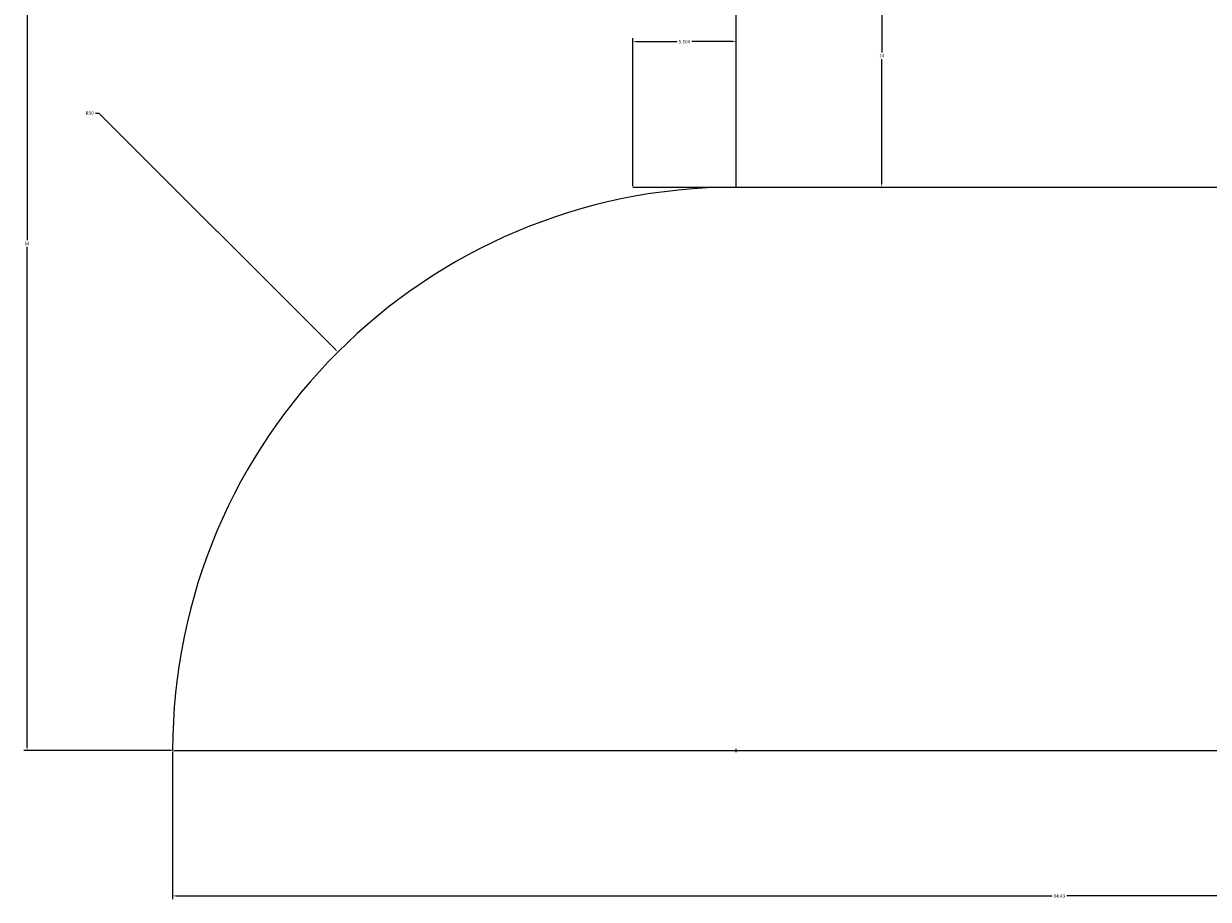
# Model space of a CAD drawing. Units: millimetres. Extents: x 118 to 244, y 285 to 440.
# Tile 1 of 4: x 118 to 181, y 285 to 331. Entities that reach past the tile are written whole.
import ezdxf

# ---------------------------------------------------------------- set-up
doc = ezdxf.new("R2010")
doc.units = ezdxf.units.MM
doc.layers.add('M-CONS', color=8, linetype='Continuous', lineweight=13)
doc.layers.add('M-DIMS', color=2, linetype='Continuous', lineweight=18)
doc.styles.get("Standard").update_dxf_attribs({"font": 'arial.ttf'})
doc.dimstyles.get("Standard").update_dxf_attribs({"dimtxt": 0.18, "dimasz": 0.18, "dimexe": 0.18, "dimexo": 0.0625, "dimgap": 0.09, "dimtad": 0, "dimtih": 1, "dimtoh": 1, "dimdec": 4, "dimzin": 0, "dimdsep": 46, "dimtxsty": 'Standard', "dimcen": 0.09, "dimadec": 0, "dimazin": 0, "dimtfac": 1, "dimtdec": 4, "dimtofl": 0, "dimtmove": 0, "dimatfit": 3, "dimfxl": 1, "dimtolj": 1, "dimtzin": 0, "dimarcsym": 0})

# ---------------------------------------------------------------- blocks, each defined once
blk = doc.blocks.new('*D1')
at = {"layer": 'Defpoints', "color": 0, "transparency": 16777216}
for p in [(219.95, 322.437), (125.524, 292.437), (219.95, 284.687)]:
    blk.add_point(p, dxfattribs=at)
at = {"layer": 'M-DIMS', "color": 0, "lineweight": -2, "transparency": 16777216}
for p, q in [((219.95, 322.374), (219.95, 284.507)), ((125.524, 292.374), (125.524, 284.507)), ((125.704, 284.687), (172.343, 284.687)), ((219.77, 284.687), (173.131, 284.687))]:
    blk.add_line(p, q, dxfattribs=at)
at = {"layer": 'M-DIMS', "color": 0, "transparency": 16777216}
for points in [[(125.704, 284.717), (125.704, 284.657), (125.524, 284.687)], [(219.77, 284.717), (219.77, 284.657), (219.95, 284.687)]]:
    blk.add_solid(points, dxfattribs=at)
at = {"layer": 'M-DIMS', "color": 0, "transparency": 16777216, "insert": (172.737, 284.687), "char_height": 0.18, "attachment_point": 5}
blk.add_mtext('\\A1;94.43', dxfattribs=at)
blk = doc.blocks.new('*D2')
at = {"layer": 'Defpoints', "color": 0, "transparency": 16777216}
for p in [(117.774, 346.437), (125.524, 346.437), (125.524, 292.437)]:
    blk.add_point(p, dxfattribs=at)
at = {"layer": 'M-DIMS', "color": 0, "lineweight": -2, "transparency": 16777216}
for p, q in [((125.462, 346.437), (117.594, 346.437)), ((117.774, 346.257), (117.774, 319.618)), ((117.774, 292.617), (117.774, 319.255)), ((125.462, 292.437), (117.594, 292.437))]:
    blk.add_line(p, q, dxfattribs=at)
at = {"layer": 'M-DIMS', "color": 0, "transparency": 16777216}
for points in [[(117.744, 346.257), (117.804, 346.257), (117.774, 346.437)], [(117.744, 292.617), (117.804, 292.617), (117.774, 292.437)]]:
    blk.add_solid(points, dxfattribs=at)
at = {"layer": 'M-DIMS', "color": 0, "transparency": 16777216, "insert": (117.774, 319.437), "char_height": 0.18, "attachment_point": 5}
blk.add_mtext('\\A1;54', dxfattribs=at)
blk = doc.blocks.new('*D6')
at = {"layer": 'Defpoints', "color": 0, "transparency": 16777216}
for p in [(155.524, 336.437), (155.524, 322.437), (163.274, 322.437)]:
    blk.add_point(p, dxfattribs=at)
at = {"layer": 'M-DIMS', "color": 0, "lineweight": -2, "transparency": 16777216}
for p, q in [((155.587, 336.437), (163.454, 336.437)), ((163.274, 336.257), (163.274, 329.617)), ((163.274, 322.617), (163.274, 329.257)), ((155.587, 322.437), (163.454, 322.437))]:
    blk.add_line(p, q, dxfattribs=at)
at = {"layer": 'M-DIMS', "color": 0, "transparency": 16777216}
for points in [[(163.244, 336.257), (163.304, 336.257), (163.274, 336.437)], [(163.244, 322.617), (163.304, 322.617), (163.274, 322.437)]]:
    blk.add_solid(points, dxfattribs=at)
at = {"layer": 'M-DIMS', "color": 0, "transparency": 16777216, "insert": (163.274, 329.437), "char_height": 0.18, "attachment_point": 5}
blk.add_mtext('\\A1;14', dxfattribs=at)
blk = doc.blocks.new('*D7')
at = {"layer": 'Defpoints', "color": 0, "transparency": 16777216}
for p in [(155.524, 330.187), (150.021, 322.437), (155.524, 322.437)]:
    blk.add_point(p, dxfattribs=at)
at = {"layer": 'M-DIMS', "color": 0, "lineweight": -2, "transparency": 16777216}
for p, q in [((150.021, 322.499), (150.021, 330.367)), ((150.201, 330.187), (152.379, 330.187)), ((155.344, 330.187), (153.166, 330.187)), ((155.524, 322.499), (155.524, 330.367))]:
    blk.add_line(p, q, dxfattribs=at)
at = {"layer": 'M-DIMS', "color": 0, "transparency": 16777216}
for points in [[(150.201, 330.217), (150.201, 330.157), (150.021, 330.187)], [(155.344, 330.217), (155.344, 330.157), (155.524, 330.187)]]:
    blk.add_solid(points, dxfattribs=at)
at = {"layer": 'M-DIMS', "color": 0, "transparency": 16777216, "insert": (152.772, 330.187), "char_height": 0.18, "attachment_point": 5}
blk.add_mtext('\\A1;5.504', dxfattribs=at)
blk = doc.blocks.new('*D10')
at = {"layer": 'Defpoints', "color": 0, "transparency": 16777216}
for p in [(235.677, 432.045), (243.427, 432.045), (125.524, 292.437)]:
    blk.add_point(p, dxfattribs=at)
at = {"layer": 'M-DIMS', "color": 0, "lineweight": -2, "transparency": 16777216}
for p, q in [((235.739, 432.045), (243.607, 432.045)), ((243.427, 431.865), (243.427, 362.423)), ((243.427, 292.617), (243.427, 362.059)), ((125.587, 292.437), (243.607, 292.437))]:
    blk.add_line(p, q, dxfattribs=at)
at = {"layer": 'M-DIMS', "color": 0, "transparency": 16777216}
for points in [[(243.397, 431.865), (243.457, 431.865), (243.427, 432.045)], [(243.397, 292.617), (243.457, 292.617), (243.427, 292.437)]]:
    blk.add_solid(points, dxfattribs=at)
at = {"layer": 'M-DIMS', "color": 0, "transparency": 16777216, "insert": (243.427, 362.241), "char_height": 0.18, "attachment_point": 5}
blk.add_mtext('\\A1;139.6', dxfattribs=at)
blk = doc.blocks.new('*D12')
at = {"layer": 'Defpoints', "color": 0, "transparency": 16777216}
for p in [(134.315, 313.655), (155.524, 292.437)]:
    blk.add_point(p, dxfattribs=at)
at = {"layer": 'M-DIMS', "color": 0, "lineweight": -2, "transparency": 16777216}
for p, q in [((121.41, 326.385), (121.59, 326.385)), ((121.59, 326.385), (134.188, 313.782)), ((155.434, 292.437), (155.614, 292.437)), ((155.524, 292.347), (155.524, 292.527))]:
    blk.add_line(p, q, dxfattribs=at)
at = {"layer": 'M-DIMS', "color": 0, "transparency": 16777216}
blk.add_solid([(134.209, 313.803), (134.167, 313.761), (134.315, 313.655)], dxfattribs=at)
at = {"layer": 'M-DIMS', "color": 0, "transparency": 16777216, "insert": (121.105, 326.385), "char_height": 0.18, "attachment_point": 5}
blk.add_mtext('\\A1;R30', dxfattribs=at)

msp = doc.modelspace()

# ---------------------------------------------------------------- linework, layer by layer
at = {"layer": 'M-CONS'}
msp.add_line((155.5241, 322.4369, 10), (155.5241, 336.4369, 10), dxfattribs=at)
msp.add_arc((155.5241, 292.4369, 10), 30, 90, 180, dxfattribs=at)
at = {"layer": 'M-CONS', "extrusion": (0, 1, 0)}
msp.add_rational_spline([(150.0206, 322.4369, 167.5697), (172.4909, 322.4369, 167.5697), (194.9611, 322.4369, 167.5697), (219.9611, 322.4369, 167.5697), (219.9611, 322.4369, 142.5697)], [1, 1, 1, 0.707106781187, 1], degree=2, knots=[0, 0, 0, 1, 1, 2.5707963, 2.5707963, 2.5707963], dxfattribs=at)

# ---------------------------------------------------------------- dimensions: what is measured, and where the dimension line sits
at = {"layer": 'M-DIMS'}
for base, p1, p2, angle, override, picture, middle in [((243.4268, 432.0445), (125.5241, 292.4369), (235.6768, 432.0445), 90, {"dimdec": 1, "dimlfac": 1, "dimrnd": 0, "dimzin": 0, "dimdsep": 46, "dimlunit": 2}, '*D10', (243.4268, 362.2407)), ((117.7741, 346.4369), (125.5241, 292.4369), (125.5241, 346.4369), 90, {"dimdec": 0, "dimlfac": 1, "dimrnd": 0, "dimzin": 0, "dimdsep": 46, "dimlunit": 2}, '*D2', (117.7741, 319.4369)), ((163.2741, 322.4369), (155.5241, 336.4369), (155.5241, 322.4369), 270, {"dimdec": 0, "dimlfac": 1, "dimrnd": 0, "dimzin": 0, "dimdsep": 46, "dimlunit": 2}, '*D6', (163.2741, 329.4369)), ((155.524113, 330.186942), (150.020608, 322.436942), (155.524113, 322.436942), 0, {"dimdec": 3, "dimlfac": 1, "dimrnd": 0, "dimzin": 0, "dimdsep": 46, "dimlunit": 2}, '*D7', (152.77236, 330.186942))]:
    dim = msp.add_linear_dim(base=base, p1=p1, p2=p2, angle=angle, dimstyle='Standard', override=override, dxfattribs=at)
    dim.commit()
    dim.dimension.update_dxf_attribs({"geometry": picture, "text_midpoint": middle})
dim = msp.add_radius_dim(center=(155.5241, 292.4369), mpoint=(134.3154, 313.6546), dimstyle='Standard', override={"dimdec": 0, "dimlfac": 1, "dimrnd": 0, "dimzin": 0, "dimdsep": 46, "dimlunit": 2}, dxfattribs=at)
dim.commit()
dim.dimension.update_dxf_attribs({"geometry": '*D12', "text_midpoint": (121.1054, 326.3852), "dimtype": 164})
dim = msp.add_linear_dim(base=(219.9501, 284.6869), p1=(125.5241, 292.4369), p2=(219.9501, 322.4369), dimstyle='Standard', override={"dimdec": 2, "dimlfac": 1, "dimrnd": 0, "dimzin": 0, "dimdsep": 46, "dimlunit": 2}, dxfattribs=at)
dim.commit()
dim.dimension.update_dxf_attribs({"geometry": '*D1', "text_midpoint": (172.7371, 284.6869)})

doc.saveas('drawing.dxf')
